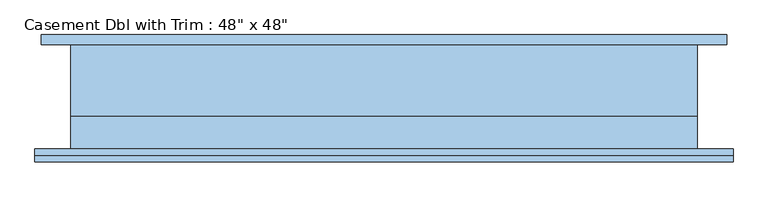
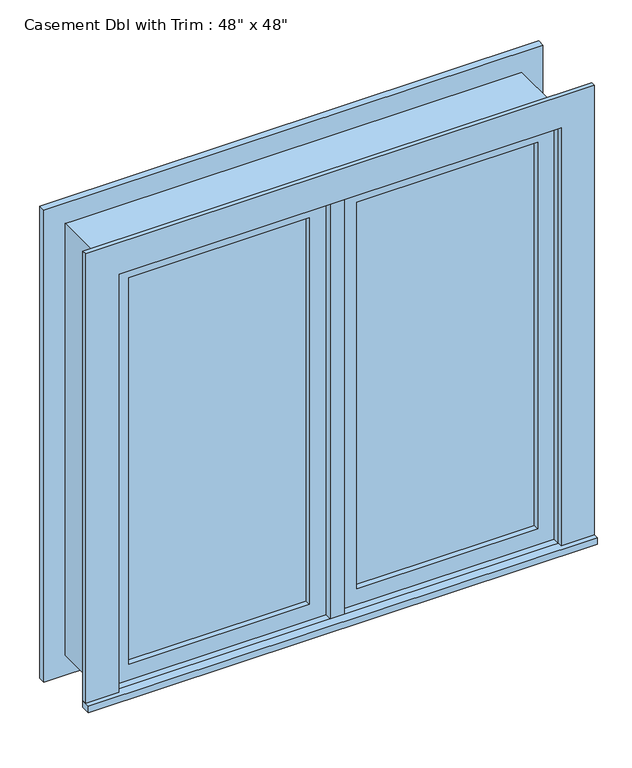
"""IFC4 building model written with IfcOpenShell, lengths in millimetres: window geometry."""

from ifc_helpers import new_model, si_unit, frame, origin, place, context, project, spatial, polyline, outline, extrude, source, transform, mapped, element, save


def window_3a1167bf(model_context):
    return source(origin(), model_context, "Body", "SweptSolid", [
        extrude(outline(polyline([(63.5, -85.725), (63.5, -73.025), (546.1, -73.025), (546.1, -85.725), (63.5, -85.725)])), frame((0.0, 0.0, 977.9), z_axis=(0.0, 0.0, 1.0), x_axis=(1.0, 0.0, 0.0)), (0.0, 0.0, 1.0), 1092.2),
        extrude(outline(polyline([(2114.55, 19.05), (933.45, 19.05), (933.45, 590.55), (2114.55, 590.55), (2114.55, 19.05)]), holes=[polyline([(2070.1, 63.5), (2070.1, 546.1), (977.9, 546.1), (977.9, 63.5), (2070.1, 63.5)])]), frame((0.0, -101.6, 0.0), z_axis=(0.0, 1.0, 0.0), x_axis=(0.0, 0.0, 1.0)), (0.0, 0.0, 1.0), 44.45),
        extrude(outline(polyline([(19.05, -57.15), (19.05, -120.65), (-19.05, -120.65), (-19.05, -57.15), (19.05, -57.15)])), frame((0.0, 0.0, 933.45), z_axis=(0.0, 0.0, 1.0), x_axis=(1.0, 0.0, 0.0)), (0.0, 0.0, 1.0), 1181.1),
        extrude(outline(polyline([(-679.45, -146.05), (-679.45, -120.65), (679.45, -120.65), (679.45, -146.05), (-679.45, -146.05)])), frame((0.0, 0.0, 914.4), z_axis=(0.0, 0.0, 1.0), x_axis=(1.0, 0.0, 0.0)), (0.0, 0.0, 1.0), 19.05),
        extrude(outline(polyline([(2114.55, -590.55), (2114.55, 590.55), (933.45, 590.55), (933.45, 679.45), (2203.45, 679.45), (2203.45, -679.45), (933.45, -679.45), (933.45, -590.55), (2114.55, -590.55)])), frame((0.0, -133.35, 0.0), z_axis=(0.0, 1.0, 0.0), x_axis=(0.0, 0.0, 1.0)), (0.0, 0.0, 1.0), 12.7),
        extrude(outline(polyline([(2190.75, 666.75), (2190.75, -666.75), (857.25, -666.75), (857.25, 666.75), (2190.75, 666.75)]), holes=[polyline([(2101.85, 577.85), (946.15, 577.85), (946.15, -577.85), (2101.85, -577.85), (2101.85, 577.85)])]), frame((0.0, 82.55, 0.0), z_axis=(0.0, 1.0, 0.0), x_axis=(0.0, 0.0, 1.0)), (0.0, 0.0, 1.0), 19.05),
        extrude(outline(polyline([(-63.5, -73.025), (-63.5, -85.725), (-546.1, -85.725), (-546.1, -73.025), (-63.5, -73.025)])), frame((0.0, 0.0, 977.9), z_axis=(0.0, 0.0, 1.0), x_axis=(1.0, 0.0, 0.0)), (0.0, 0.0, 1.0), 1092.2),
        extrude(outline(polyline([(2114.55, -590.55), (933.45, -590.55), (933.45, -19.05), (2114.55, -19.05), (2114.55, -590.55)]), holes=[polyline([(2070.1, -546.1), (2070.1, -63.5), (977.9, -63.5), (977.9, -546.1), (2070.1, -546.1)])]), frame((0.0, -101.6, 0.0), z_axis=(0.0, 1.0, 0.0), x_axis=(0.0, 0.0, 1.0)), (0.0, 0.0, 1.0), 44.45),
        extrude(outline(polyline([(2133.6, -609.6), (914.4, -609.6), (914.4, 609.6), (2133.6, 609.6), (2133.6, -609.6)]), holes=[polyline([(2101.85, -577.85), (2101.85, 577.85), (946.15, 577.85), (946.15, -577.85), (2101.85, -577.85)])]), frame((0.0, -57.15, 0.0), z_axis=(0.0, 1.0, 0.0), x_axis=(0.0, 0.0, 1.0)), (0.0, 0.0, 1.0), 139.7),
        extrude(outline(polyline([(2133.6, 609.6), (2133.6, -609.6), (914.4, -609.6), (914.4, 609.6), (2133.6, 609.6)]), holes=[polyline([(2114.55, 590.55), (933.45, 590.55), (933.45, -590.55), (2114.55, -590.55), (2114.55, 590.55)])]), frame((0.0, -120.65, 0.0), z_axis=(0.0, 1.0, 0.0), x_axis=(0.0, 0.0, 1.0)), (0.0, 0.0, 1.0), 63.5),
    ])


if __name__ == "__main__":
    model = new_model("IFC4")
    model_context = context("Model", 3, world=origin())
    ifc_project = project(units=[si_unit("LENGTHUNIT", "METRE", prefix="MILLI")], contexts=[model_context])
    site = spatial("IfcSite", under=ifc_project)
    building = spatial("IfcBuilding", under=site)
    placement = place(None, origin())
    window_shape = window_3a1167bf(model_context)
    element("IfcWindow", 1, ObjectType="Casement Dbl with Trim : 48\" x 48\"", at=placement, inside=building, context=model_context, shape_type="MappedRepresentation", body=[
        mapped(window_shape, transform((0.0, 0.0, 0.0), x_axis=(1.0, 0.0, 0.0), y_axis=(0.0, 1.0, 0.0), z_axis=(0.0, 0.0, 1.0))),
    ])
    save(model, "model.ifc")

# Revit data of these elements
# Type "Casement Dbl with Trim : 48\" x 48\""
#   Type Mark = "10"
#   Construction Type Id = "GSP4R"
#   Assembly Code = "B2020100"
#   Analytic Construction = "1/8 in Pilkington single glazing"
#   Visual Light Transmittance = 0.9
#   Thermal Resistance (R) = 1.53941 (h·ft²·°F)/BTU
#   Solar Heat Gain Coefficient = 0.78
#   Heat Transfer Coefficient (U) = 0.6496 BTU/(h·ft²·°F)
#   Height = 4' - 0"
#   Default Sill Height = 3' - 0"
#   Trim Projection - Ext. = 0' - 0 1/2"
#   Trim Projection - Int. = 0' - 0 3/4"
#   Trim Width - Exterior = 0' - 3 1/2"
#   Trim Width - Interior = 0' - 3 1/2"
#   Width = 4' - 0"
#   Window Inset = 0' - 0 3/4"
#   Define Thermal Properties by = 1
#   Glass Pane Material = Glass
#   Sash Material = Sash
#   Trim Exterior Material = Trim
#   Trim Interior Material = Trim
#   Wall Closure = (empty or 0)
# Element 1 (IfcWindow, "Casement Dbl with Trim : 48\" x 48\"")
#   Materials on its faces: "Sash", "Trim", "Glass"
# Materials
#   "Glass": class "Glass", colour RGB 0 128 192, transparency 0.75, Description = "Soda Lime Glass", Cost = 0
#   "Sash": class "Wood", colour RGB 224 178 126, transparency 0
#   "Trim": class "Wood", colour RGB 224 178 126, transparency 0
